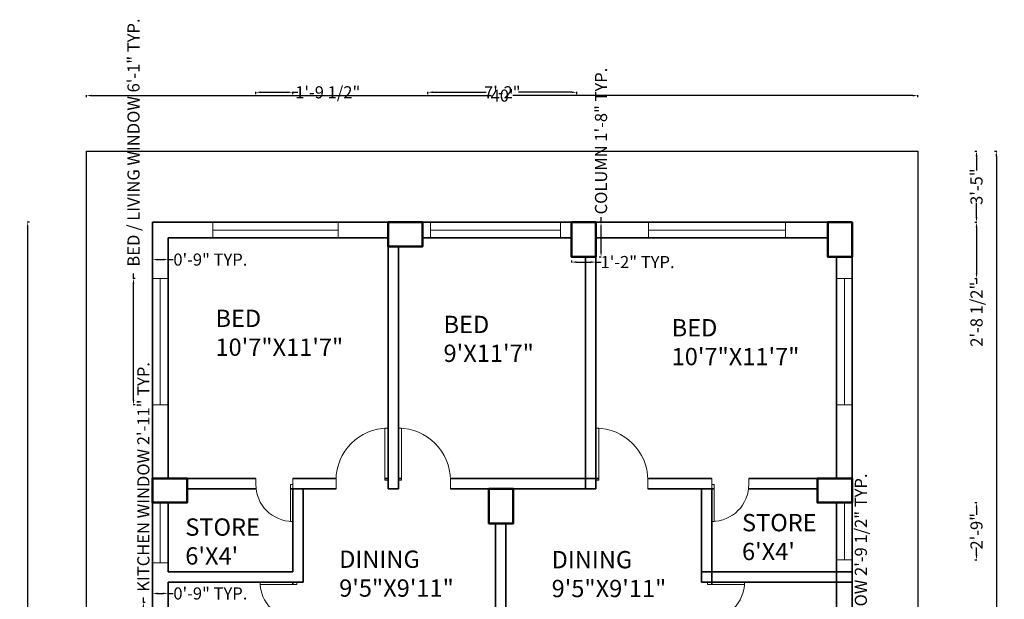
# Model space of a CAD drawing. Units: inches. Extents: x -78 to 529, y -573 to 148.
# Tile 2 of 2: x -78 to 491, y -187 to 148. Entities that reach past the tile are written whole.
import ezdxf

# ---------------------------------------------------------------- set-up
doc = ezdxf.new("R2010")
doc.units = ezdxf.units.IN
doc.header["$MEASUREMENT"] = 0
for name, color, linetype, lineweight in [('A-ANNO-DIMS', 2, 'Continuous', 18), ('A-AREA-IDEN', 5, 'Continuous', 18), ('A-COLS', 1, 'Continuous', 50), ('A-DOOR', 3, 'Continuous', 18), ('A-GLAZ', 4, 'Continuous', 18), ('A-WALL', 7, 'Continuous', 35), ('C-PROP', 8, 'Continuous', 25)]:
    doc.layers.add(name, color=color, linetype=linetype, lineweight=lineweight)
doc.styles.get("Standard").update_dxf_attribs({"font": 'arial.ttf'})
doc.dimstyles.get("Standard").update_dxf_attribs({"dimtxt": 7, "dimasz": 3, "dimexe": 0.18, "dimexo": 0.0625, "dimgap": 0.09, "dimtad": 0, "dimdec": 0, "dimzin": 0, "dimdsep": 46, "dimlunit": 3, "dimtxsty": 'Standard', "dimcen": 0.09, "dimadec": 0, "dimazin": 0, "dimtfac": 1, "dimtdec": 0, "dimtofl": 0, "dimtmove": 0, "dimatfit": 3, "dimfxl": 1, "dimfxlon": 1, "dimtolj": 1, "dimtzin": 0, "dimarcsym": 0})

# ---------------------------------------------------------------- blocks, each defined once
blk = doc.blocks.new('*U2')
for p, q in [((0, 0), (0, -5)), ((30, 0), (30, -5))]:
    blk.add_line(p, q)
blk.add_lwpolyline([(0, 0), (0, 30), (1.75, 30), (1.75, 0)], close=True)
blk.add_arc((0, 0), 30, 0, 90)
blk = doc.blocks.new('*D3')
at = {"layer": 'A-ANNO-DIMS', "color": 0, "lineweight": -2, "transparency": 16777216}
for p, q in [((-39.22, 102.81), (-39.22, 103.99)), ((-36.22, 103.81), (194.61, 103.81)), ((437.78, 103.81), (206.95, 103.81)), ((440.78, 102.81), (440.78, 103.99))]:
    blk.add_line(p, q, dxfattribs=at)
at = {"layer": 'A-ANNO-DIMS', "color": 0, "transparency": 16777216}
for points in [[(-36.22, 104.31), (-36.22, 103.31), (-39.22, 103.81)], [(437.78, 104.31), (437.78, 103.31), (440.78, 103.81)]]:
    blk.add_solid(points, dxfattribs=at)
at = {"layer": 'Defpoints', "color": 0, "transparency": 16777216}
for p in [(-39.22, 103.81), (-39.22, 71.78), (440.78, 71.78)]:
    blk.add_point(p, dxfattribs=at)
at = {"layer": 'A-ANNO-DIMS', "color": 0, "transparency": 16777216, "insert": (200.78, 103.81), "char_height": 7, "attachment_point": 5}
blk.add_mtext("\\A1;40'", dxfattribs=at)
blk = doc.blocks.new('*D4')
at = {"layer": 'A-ANNO-DIMS', "color": 0, "lineweight": -2, "transparency": 16777216}
for p, q in [((485.19, 71.78), (486.37, 71.78)), ((486.19, 68.78), (486.19, -222.19)), ((486.19, -525.22), (486.19, -234.25)), ((485.19, -528.22), (486.37, -528.22))]:
    blk.add_line(p, q, dxfattribs=at)
at = {"layer": 'A-ANNO-DIMS', "color": 0, "transparency": 16777216}
for points in [[(485.69, 68.78), (486.69, 68.78), (486.19, 71.78)], [(485.69, -525.22), (486.69, -525.22), (486.19, -528.22)]]:
    blk.add_solid(points, dxfattribs=at)
at = {"layer": 'Defpoints', "color": 0, "transparency": 16777216}
for p in [(440.78, 71.78), (440.78, -528.22), (486.19, -528.22)]:
    blk.add_point(p, dxfattribs=at)
at = {"layer": 'A-ANNO-DIMS', "color": 0, "transparency": 16777216, "insert": (486.19, -228.22), "char_height": 7, "attachment_point": 5, "rotation": 90}
blk.add_mtext("\\A1;50'", dxfattribs=at)
blk = doc.blocks.new('COLUMN-14X20')
blk.add_lwpolyline([(0, 20), (14, 20), (14, 0), (0, 0)], close=True)
blk = doc.blocks.new('WIN-BED-LIVING')
for p, q in [((0, 73.06), (9, 73.06)), ((4.5, 0), (4.5, 73.06)), ((0, 0), (9, 0))]:
    blk.add_line(p, q)
blk = doc.blocks.new('*D10')
at = {"layer": 'A-ANNO-DIMS', "color": 0, "lineweight": -2, "transparency": 16777216}
for p, q in [((256.91, 30.61), (258.09, 30.61)), ((257.91, 30.61), (257.91, 33.61)), ((257.91, 13.61), (257.91, 27.61)), ((256.91, 10.61), (258.09, 10.61))]:
    blk.add_line(p, q, dxfattribs=at)
at = {"layer": 'A-ANNO-DIMS', "color": 0, "transparency": 16777216}
for points in [[(257.41, 27.61), (258.41, 27.61), (257.91, 30.61)], [(257.41, 13.61), (258.41, 13.61), (257.91, 10.61)]]:
    blk.add_solid(points, dxfattribs=at)
at = {"layer": 'Defpoints', "color": 0, "transparency": 16777216}
for p in [(254.91, 30.61), (257.91, 30.61), (254.91, 10.61)]:
    blk.add_point(p, dxfattribs=at)
at = {"layer": 'A-ANNO-DIMS', "color": 0, "transparency": 16777216, "insert": (257.91, 77.54), "char_height": 7, "attachment_point": 5, "rotation": 90}
blk.add_mtext('\\A1;COLUMN 1\'-8" TYP.', dxfattribs=at)
blk = doc.blocks.new('*D11')
at = {"layer": 'A-ANNO-DIMS', "color": 0, "lineweight": -2, "transparency": 16777216}
for p, q in [((240.91, 8.61), (240.91, 7.43)), ((243.91, 7.61), (251.91, 7.61)), ((254.91, 8.61), (254.91, 7.43)), ((254.91, 7.61), (257.91, 7.61))]:
    blk.add_line(p, q, dxfattribs=at)
at = {"layer": 'A-ANNO-DIMS', "color": 0, "transparency": 16777216}
for points in [[(243.91, 8.11), (243.91, 7.11), (240.91, 7.61)], [(251.91, 8.11), (251.91, 7.11), (254.91, 7.61)]]:
    blk.add_solid(points, dxfattribs=at)
at = {"layer": 'Defpoints', "color": 0, "transparency": 16777216}
for p in [(240.91, 10.61), (254.91, 10.61), (254.91, 7.61)]:
    blk.add_point(p, dxfattribs=at)
at = {"layer": 'A-ANNO-DIMS', "color": 0, "transparency": 16777216, "insert": (279.01, 7.61), "char_height": 7, "attachment_point": 5}
blk.add_mtext('\\A1;1\'-2" TYP.', dxfattribs=at)
blk = doc.blocks.new('*D12')
at = {"layer": 'A-ANNO-DIMS', "color": 0, "lineweight": -2, "transparency": 16777216}
for p, q in [((-12.05, -1.91), (-12.05, 1.09)), ((-11.05, -1.91), (-12.23, -1.91)), ((-12.05, -71.97), (-12.05, -4.91)), ((-11.05, -74.97), (-12.23, -74.97))]:
    blk.add_line(p, q, dxfattribs=at)
at = {"layer": 'A-ANNO-DIMS', "color": 0, "transparency": 16777216}
for points in [[(-12.55, -4.91), (-11.55, -4.91), (-12.05, -1.91)], [(-12.55, -71.97), (-11.55, -71.97), (-12.05, -74.97)]]:
    blk.add_solid(points, dxfattribs=at)
at = {"layer": 'Defpoints', "color": 0, "transparency": 16777216}
for p in [(-12.05, -1.91), (-1.09, -1.91), (-1.09, -74.97)]:
    blk.add_point(p, dxfattribs=at)
at = {"layer": 'A-ANNO-DIMS', "color": 0, "transparency": 16777216, "insert": (-12.05, 76.69), "char_height": 7, "attachment_point": 5, "rotation": 90}
blk.add_mtext('\\A1;BED / LIVING WINDOW 6\'-1" TYP.', dxfattribs=at)
blk = doc.blocks.new('*D13')
at = {"layer": 'A-ANNO-DIMS', "color": 0, "lineweight": -2, "transparency": 16777216}
for p, q in [((-1.09, 8.05), (-1.09, 9.23)), ((1.91, 9.05), (4.91, 9.05)), ((7.91, 8.05), (7.91, 9.23)), ((7.91, 9.05), (10.91, 9.05))]:
    blk.add_line(p, q, dxfattribs=at)
at = {"layer": 'A-ANNO-DIMS', "color": 0, "transparency": 16777216}
for points in [[(1.91, 9.55), (1.91, 8.55), (-1.09, 9.05)], [(4.91, 9.55), (4.91, 8.55), (7.91, 9.05)]]:
    blk.add_solid(points, dxfattribs=at)
at = {"layer": 'Defpoints', "color": 0, "transparency": 16777216}
for p in [(7.91, 9.05), (-1.09, -1.91), (7.91, -1.91)]:
    blk.add_point(p, dxfattribs=at)
at = {"layer": 'A-ANNO-DIMS', "color": 0, "transparency": 16777216, "insert": (32.34, 9.05), "char_height": 7, "attachment_point": 5}
blk.add_mtext('\\A1;0\'-9" TYP.', dxfattribs=at)
blk = doc.blocks.new('*D16')
at = {"layer": 'A-ANNO-DIMS', "color": 0, "lineweight": -2, "transparency": 16777216}
for p, q in [((-6.35, -189.15), (-6.35, -186.15)), ((-5.35, -189.15), (-6.53, -189.15)), ((-6.35, -221.25), (-6.35, -192.15)), ((-5.35, -224.25), (-6.53, -224.25))]:
    blk.add_line(p, q, dxfattribs=at)
at = {"layer": 'A-ANNO-DIMS', "color": 0, "transparency": 16777216}
for points in [[(-6.85, -192.15), (-5.85, -192.15), (-6.35, -189.15)], [(-6.85, -221.25), (-5.85, -221.25), (-6.35, -224.25)]]:
    blk.add_solid(points, dxfattribs=at)
at = {"layer": 'Defpoints', "color": 0, "transparency": 16777216}
for p in [(-6.35, -189.15), (-1.09, -189.15), (-1.09, -224.25)]:
    blk.add_point(p, dxfattribs=at)
at = {"layer": 'A-ANNO-DIMS', "color": 0, "transparency": 16777216, "insert": (-6.35, -116.53), "char_height": 7, "attachment_point": 5, "rotation": 90}
blk.add_mtext('\\A1;KITCHEN WINDOW 2\'-11" TYP.', dxfattribs=at)
blk = doc.blocks.new('*D17')
at = {"layer": 'A-ANNO-DIMS', "color": 0, "lineweight": -2, "transparency": 16777216}
for p, q in [((-1.09, -184.89), (-1.09, -183.71)), ((1.91, -183.89), (4.91, -183.89)), ((7.91, -184.89), (7.91, -183.71)), ((7.91, -183.89), (10.91, -183.89))]:
    blk.add_line(p, q, dxfattribs=at)
at = {"layer": 'A-ANNO-DIMS', "color": 0, "transparency": 16777216}
for points in [[(1.91, -183.39), (1.91, -184.39), (-1.09, -183.89)], [(4.91, -183.39), (4.91, -184.39), (7.91, -183.89)]]:
    blk.add_solid(points, dxfattribs=at)
at = {"layer": 'Defpoints', "color": 0, "transparency": 16777216}
for p in [(7.91, -183.89), (-1.09, -189.15), (7.91, -189.15)]:
    blk.add_point(p, dxfattribs=at)
at = {"layer": 'A-ANNO-DIMS', "color": 0, "transparency": 16777216, "insert": (32.34, -183.89), "char_height": 7, "attachment_point": 5}
blk.add_mtext('\\A1;0\'-9" TYP.', dxfattribs=at)
blk = doc.blocks.new('*D18')
at = {"layer": 'A-ANNO-DIMS', "color": 0, "lineweight": -2, "transparency": 16777216}
for p, q in [((407.95, -256.39), (407.95, -253.39)), ((406.95, -256.39), (408.13, -256.39)), ((407.95, -286.96), (407.95, -259.39)), ((406.95, -289.96), (408.13, -289.96))]:
    blk.add_line(p, q, dxfattribs=at)
at = {"layer": 'A-ANNO-DIMS', "color": 0, "transparency": 16777216}
for points in [[(407.45, -259.39), (408.45, -259.39), (407.95, -256.39)], [(407.45, -286.96), (408.45, -286.96), (407.95, -289.96)]]:
    blk.add_solid(points, dxfattribs=at)
at = {"layer": 'Defpoints', "color": 0, "transparency": 16777216}
for p in [(402.91, -256.39), (407.95, -256.39), (402.91, -289.96)]:
    blk.add_point(p, dxfattribs=at)
at = {"layer": 'A-ANNO-DIMS', "color": 0, "transparency": 16777216, "insert": (407.95, -182.44), "char_height": 7, "attachment_point": 5, "rotation": 90}
blk.add_mtext('\\A1;TOILET WINDOW 2\'-9 1/2" TYP.', dxfattribs=at)
blk = doc.blocks.new('*D21')
at = {"layer": 'A-ANNO-DIMS', "color": 0, "lineweight": -2, "transparency": 16777216}
for p, q in [((-72.17, 30.61), (-73.35, 30.61)), ((-73.17, 27.61), (-73.17, -212.14)), ((-73.17, -476.39), (-73.17, -236.65)), ((-72.17, -479.39), (-73.35, -479.39))]:
    blk.add_line(p, q, dxfattribs=at)
at = {"layer": 'A-ANNO-DIMS', "color": 0, "transparency": 16777216}
for points in [[(-73.67, 27.61), (-72.67, 27.61), (-73.17, 30.61)], [(-73.67, -476.39), (-72.67, -476.39), (-73.17, -479.39)]]:
    blk.add_solid(points, dxfattribs=at)
at = {"layer": 'Defpoints', "color": 0, "transparency": 16777216}
for p in [(-73.17, 30.61), (-1.09, 30.61), (-1.09, -479.39)]:
    blk.add_point(p, dxfattribs=at)
at = {"layer": 'A-ANNO-DIMS', "color": 0, "transparency": 16777216, "insert": (-73.17, -224.39), "char_height": 7, "attachment_point": 5, "rotation": 90}
blk.add_mtext('\\A1;42\'-6"', dxfattribs=at)
blk = doc.blocks.new('*D23')
at = {"layer": 'A-ANNO-DIMS', "color": 0, "lineweight": -2, "transparency": 16777216}
for p, q in [((473.73, 71.78), (474.91, 71.78)), ((474.73, 68.78), (474.73, 60.59)), ((474.73, 33.61), (474.73, 41.8)), ((473.73, 30.61), (474.91, 30.61))]:
    blk.add_line(p, q, dxfattribs=at)
at = {"layer": 'A-ANNO-DIMS', "color": 0, "transparency": 16777216}
for points in [[(474.23, 68.78), (475.23, 68.78), (474.73, 71.78)], [(474.23, 33.61), (475.23, 33.61), (474.73, 30.61)]]:
    blk.add_solid(points, dxfattribs=at)
at = {"layer": 'Defpoints', "color": 0, "transparency": 16777216}
for p in [(440.78, 71.78), (402.91, 30.61), (474.73, 30.61)]:
    blk.add_point(p, dxfattribs=at)
at = {"layer": 'A-ANNO-DIMS', "color": 0, "transparency": 16777216, "insert": (474.73, 51.19), "char_height": 7, "attachment_point": 5, "rotation": 90}
blk.add_mtext('\\A1;3\'-5"', dxfattribs=at)
blk = doc.blocks.new('*D24')
at = {"layer": 'A-ANNO-DIMS', "color": 0, "lineweight": -2, "transparency": 16777216}
for p, q in [((157.91, 104.73), (157.91, 105.91)), ((160.91, 105.73), (191.55, 105.73)), ((240.91, 105.73), (210.28, 105.73)), ((243.91, 104.73), (243.91, 105.91))]:
    blk.add_line(p, q, dxfattribs=at)
at = {"layer": 'A-ANNO-DIMS', "color": 0, "transparency": 16777216}
for points in [[(160.91, 106.23), (160.91, 105.23), (157.91, 105.73)], [(240.91, 106.23), (240.91, 105.23), (243.91, 105.73)]]:
    blk.add_solid(points, dxfattribs=at)
at = {"layer": 'Defpoints', "color": 0, "transparency": 16777216}
for p in [(243.91, 105.73), (157.91, -433.39), (243.91, -433.39)]:
    blk.add_point(p, dxfattribs=at)
at = {"layer": 'A-ANNO-DIMS', "color": 0, "transparency": 16777216, "insert": (200.91, 105.73), "char_height": 7, "attachment_point": 5}
blk.add_mtext('\\A1;7\'-2"', dxfattribs=at)
blk = doc.blocks.new('*D28')
at = {"layer": 'A-ANNO-DIMS', "color": 0, "lineweight": -2, "transparency": 16777216}
for p, q in [((58.59, 104.73), (58.59, 105.91)), ((61.59, 105.73), (76.91, 105.73)), ((79.91, 104.73), (79.91, 105.91)), ((79.91, 105.73), (82.91, 105.73))]:
    blk.add_line(p, q, dxfattribs=at)
at = {"layer": 'A-ANNO-DIMS', "color": 0, "transparency": 16777216}
for points in [[(61.59, 106.23), (61.59, 105.23), (58.59, 105.73)], [(76.91, 106.23), (76.91, 105.23), (79.91, 105.73)]]:
    blk.add_solid(points, dxfattribs=at)
at = {"layer": 'Defpoints', "color": 0, "transparency": 16777216}
for p in [(79.91, 105.73), (58.59, -117.39), (79.91, -117.39)]:
    blk.add_point(p, dxfattribs=at)
at = {"layer": 'A-ANNO-DIMS', "color": 0, "transparency": 16777216, "insert": (100.13, 105.73), "char_height": 7, "attachment_point": 5}
blk.add_mtext('\\A1;1\'-9 1/2"', dxfattribs=at)
blk = doc.blocks.new('*D29')
at = {"layer": 'A-ANNO-DIMS', "color": 0, "lineweight": -2, "transparency": 16777216}
for p, q in [((7.91, -561.17), (7.91, -562.35)), ((10.91, -562.17), (11.34, -562.17)), ((30.68, -562.17), (30.25, -562.17)), ((33.68, -561.17), (33.68, -562.35))]:
    blk.add_line(p, q, dxfattribs=at)
at = {"layer": 'A-ANNO-DIMS', "color": 0, "transparency": 16777216}
for points in [[(10.91, -561.67), (10.91, -562.67), (7.91, -562.17)], [(30.68, -561.67), (30.68, -562.67), (33.68, -562.17)]]:
    blk.add_solid(points, dxfattribs=at)
at = {"layer": 'Defpoints', "color": 0, "transparency": 16777216}
for p in [(7.91, 21.61), (33.68, 21.61), (33.68, -562.17)]:
    blk.add_point(p, dxfattribs=at)
at = {"layer": 'A-ANNO-DIMS', "color": 0, "transparency": 16777216, "insert": (20.79, -562.17), "char_height": 7, "attachment_point": 5}
blk.add_mtext('\\A1;2\'-2"', dxfattribs=at)
blk = doc.blocks.new('*D30')
at = {"layer": 'A-ANNO-DIMS', "color": 0, "lineweight": -2, "transparency": 16777216}
for p, q in [((33.68, -561.17), (33.68, -562.35)), ((36.68, -562.17), (52.37, -562.17)), ((103.2, -562.17), (87.51, -562.17)), ((106.2, -561.17), (106.2, -562.35))]:
    blk.add_line(p, q, dxfattribs=at)
at = {"layer": 'A-ANNO-DIMS', "color": 0, "transparency": 16777216}
for points in [[(36.68, -561.67), (36.68, -562.67), (33.68, -562.17)], [(103.2, -561.67), (103.2, -562.67), (106.2, -562.17)]]:
    blk.add_solid(points, dxfattribs=at)
at = {"layer": 'Defpoints', "color": 0, "transparency": 16777216}
for p in [(33.68, 21.61), (106.2, 21.61), (106.2, -562.17)]:
    blk.add_point(p, dxfattribs=at)
at = {"layer": 'A-ANNO-DIMS', "color": 0, "transparency": 16777216, "insert": (69.94, -562.17), "char_height": 7, "attachment_point": 5}
blk.add_mtext('\\A1;6\'-0 1/2"', dxfattribs=at)
blk = doc.blocks.new('*D31')
at = {"layer": 'A-ANNO-DIMS', "color": 0, "lineweight": -2, "transparency": 16777216}
for p, q in [((134.91, -561.17), (134.91, -562.35)), ((137.91, -562.17), (156.38, -562.17)), ((159.38, -561.17), (159.38, -562.35)), ((159.38, -562.17), (162.38, -562.17))]:
    blk.add_line(p, q, dxfattribs=at)
at = {"layer": 'A-ANNO-DIMS', "color": 0, "transparency": 16777216}
for points in [[(137.91, -561.67), (137.91, -562.67), (134.91, -562.17)], [(156.38, -561.67), (156.38, -562.67), (159.38, -562.17)]]:
    blk.add_solid(points, dxfattribs=at)
at = {"layer": 'Defpoints', "color": 0, "transparency": 16777216}
for p in [(134.91, 30.61), (159.38, 21.61), (159.38, -562.17)]:
    blk.add_point(p, dxfattribs=at)
at = {"layer": 'A-ANNO-DIMS', "color": 0, "transparency": 16777216, "insert": (179.99, -562.17), "char_height": 7, "attachment_point": 5}
blk.add_mtext('\\A1;2\'-0 1/2"', dxfattribs=at)
blk = doc.blocks.new('*D32')
at = {"layer": 'A-ANNO-DIMS', "color": 0, "lineweight": -2, "transparency": 16777216}
for p, q in [((159.38, -561.17), (159.38, -562.35)), ((162.38, -562.17), (187.51, -562.17)), ((231.46, -562.17), (206.34, -562.17)), ((234.46, -561.17), (234.46, -562.35))]:
    blk.add_line(p, q, dxfattribs=at)
at = {"layer": 'A-ANNO-DIMS', "color": 0, "transparency": 16777216}
for points in [[(162.38, -561.67), (162.38, -562.67), (159.38, -562.17)], [(231.46, -561.67), (231.46, -562.67), (234.46, -562.17)]]:
    blk.add_solid(points, dxfattribs=at)
at = {"layer": 'Defpoints', "color": 0, "transparency": 16777216}
for p in [(159.38, 21.61), (234.46, 21.61), (234.46, -562.17)]:
    blk.add_point(p, dxfattribs=at)
at = {"layer": 'A-ANNO-DIMS', "color": 0, "transparency": 16777216, "insert": (196.92, -562.17), "char_height": 7, "attachment_point": 5}
blk.add_mtext('\\A1;6\'-3"', dxfattribs=at)
blk = doc.blocks.new('*D33')
at = {"layer": 'A-ANNO-DIMS', "color": 0, "lineweight": -2, "transparency": 16777216}
for p, q in [((364.5, -561.17), (364.5, -562.35)), ((367.5, -562.17), (385.91, -562.17)), ((388.91, -561.17), (388.91, -562.35)), ((388.91, -562.17), (391.91, -562.17))]:
    blk.add_line(p, q, dxfattribs=at)
at = {"layer": 'A-ANNO-DIMS', "color": 0, "transparency": 16777216}
for points in [[(367.5, -561.67), (367.5, -562.67), (364.5, -562.17)], [(385.91, -561.67), (385.91, -562.67), (388.91, -562.17)]]:
    blk.add_solid(points, dxfattribs=at)
at = {"layer": 'Defpoints', "color": 0, "transparency": 16777216}
for p in [(364.5, 21.61), (388.91, 10.61), (388.91, -562.17)]:
    blk.add_point(p, dxfattribs=at)
at = {"layer": 'A-ANNO-DIMS', "color": 0, "transparency": 16777216, "insert": (409.52, -562.17), "char_height": 7, "attachment_point": 5}
blk.add_mtext('\\A1;2\'-0 1/2"', dxfattribs=at)
blk = doc.blocks.new('*D34')
at = {"layer": 'A-ANNO-DIMS', "color": 0, "lineweight": -2, "transparency": 16777216}
for p, q in [((285.28, -561.17), (285.28, -562.35)), ((288.28, -562.17), (315.48, -562.17)), ((361.5, -562.17), (334.3, -562.17)), ((364.5, -561.17), (364.5, -562.35))]:
    blk.add_line(p, q, dxfattribs=at)
at = {"layer": 'A-ANNO-DIMS', "color": 0, "transparency": 16777216}
for points in [[(288.28, -561.67), (288.28, -562.67), (285.28, -562.17)], [(361.5, -561.67), (361.5, -562.67), (364.5, -562.17)]]:
    blk.add_solid(points, dxfattribs=at)
at = {"layer": 'Defpoints', "color": 0, "transparency": 16777216}
for p in [(285.28, 21.61), (364.5, 21.61), (364.5, -562.17)]:
    blk.add_point(p, dxfattribs=at)
at = {"layer": 'A-ANNO-DIMS', "color": 0, "transparency": 16777216, "insert": (324.89, -562.17), "char_height": 7, "attachment_point": 5}
blk.add_mtext('\\A1;6\'-7"', dxfattribs=at)
blk = doc.blocks.new('*D35')
at = {"layer": 'A-ANNO-DIMS', "color": 0, "lineweight": -2, "transparency": 16777216}
for p, q in [((473.73, 30.61), (474.91, 30.61)), ((474.73, 27.61), (474.73, 1.09)), ((473.73, -1.91), (474.91, -1.91)), ((474.73, -1.91), (474.73, -4.91))]:
    blk.add_line(p, q, dxfattribs=at)
at = {"layer": 'A-ANNO-DIMS', "color": 0, "transparency": 16777216}
for points in [[(474.23, 27.61), (475.23, 27.61), (474.73, 30.61)], [(474.23, 1.09), (475.23, 1.09), (474.73, -1.91)]]:
    blk.add_solid(points, dxfattribs=at)
at = {"layer": 'Defpoints', "color": 0, "transparency": 16777216}
for p in [(402.91, 30.61), (402.91, -1.91), (474.73, -1.91)]:
    blk.add_point(p, dxfattribs=at)
at = {"layer": 'A-ANNO-DIMS', "color": 0, "transparency": 16777216, "insert": (474.73, -22.52), "char_height": 7, "attachment_point": 5, "rotation": 90}
blk.add_mtext('\\A1;2\'-8 1/2"', dxfattribs=at)
blk = doc.blocks.new('*D37')
at = {"layer": 'A-ANNO-DIMS', "color": 0, "lineweight": -2, "transparency": 16777216}
for p, q in [((473.73, -131.41), (474.91, -131.41)), ((474.73, -134.41), (474.73, -138.48)), ((474.73, -161.46), (474.73, -157.39)), ((473.73, -164.46), (474.91, -164.46))]:
    blk.add_line(p, q, dxfattribs=at)
at = {"layer": 'A-ANNO-DIMS', "color": 0, "transparency": 16777216}
for points in [[(474.23, -134.41), (475.23, -134.41), (474.73, -131.41)], [(474.23, -161.46), (475.23, -161.46), (474.73, -164.46)]]:
    blk.add_solid(points, dxfattribs=at)
at = {"layer": 'Defpoints', "color": 0, "transparency": 16777216}
for p in [(402.91, -131.41), (402.91, -164.46), (474.73, -164.46)]:
    blk.add_point(p, dxfattribs=at)
at = {"layer": 'A-ANNO-DIMS', "color": 0, "transparency": 16777216, "insert": (474.73, -147.94), "char_height": 7, "attachment_point": 5, "rotation": 90}
blk.add_mtext('\\A1;2\'-9"', dxfattribs=at)
blk = doc.blocks.new('*D38')
at = {"layer": 'A-ANNO-DIMS', "color": 0, "lineweight": -2, "transparency": 16777216}
for p, q in [((131.91, -562.17), (128.91, -562.17)), ((134.91, -561.17), (134.91, -562.35)), ((140.91, -561.17), (140.91, -562.35)), ((143.91, -562.17), (146.91, -562.17))]:
    blk.add_line(p, q, dxfattribs=at)
at = {"layer": 'A-ANNO-DIMS', "color": 0, "transparency": 16777216}
for points in [[(131.91, -561.67), (131.91, -562.67), (134.91, -562.17)], [(143.91, -561.67), (143.91, -562.67), (140.91, -562.17)]]:
    blk.add_solid(points, dxfattribs=at)
at = {"layer": 'Defpoints', "color": 0, "transparency": 16777216}
for p in [(134.91, -123.39), (140.91, -123.39), (140.91, -562.17)]:
    blk.add_point(p, dxfattribs=at)
at = {"layer": 'A-ANNO-DIMS', "color": 0, "transparency": 16777216, "insert": (156.31, -562.17), "char_height": 7, "attachment_point": 5}
blk.add_mtext('\\A1;0\'-6"', dxfattribs=at)

msp = doc.modelspace()

# ---------------------------------------------------------------- linework, layer by layer
at = {"layer": 'A-GLAZ'}
for p, q in [((33.68, 30.61), (33.68, 21.61)), ((106.2, 30.61), (106.2, 21.61)), ((159.38, 30.61), (159.38, 21.61)), ((234.46, 30.61), (234.46, 21.61)), ((285.28, 30.61), (285.28, 21.61)), ((364.5, 30.61), (364.5, 21.61)), ((33.68, 26.11), (106.2, 26.11)), ((159.38, 26.11), (234.46, 26.11)), ((285.28, 26.11), (364.5, 26.11)), ((3.41, -131.39), (3.41, -166.28)), ((398.41, -131.41), (398.41, -164.46)), ((393.91, -164.46), (402.91, -164.46)), ((-1.09, -166.28), (7.91, -166.28))]:
    msp.add_line(p, q, dxfattribs=at)
at = {"layer": 'A-WALL'}
for p, q in [((-1.09, 30.61), (402.91, 30.61)), ((-1.09, 30.61), (-1.09, -439.39)), ((402.91, 30.61), (402.91, -439.39)), ((7.91, 21.61), (134.91, 21.61)), ((7.91, 21.61), (7.91, -117.39)), ((134.91, 21.61), (134.91, -123.39)), ((154.91, 21.61), (240.91, 21.61)), ((254.91, 21.61), (254.91, -123.39)), ((254.91, 21.61), (388.91, 21.61)), ((140.91, 16.61), (140.91, -123.39)), ((248.91, 10.61), (248.91, -123.39)), ((393.91, 10.61), (393.91, -117.39)), ((7.91, -117.39), (58.59, -117.39)), ((79.91, -117.39), (104.93, -117.39)), ((133.16, -117.39), (134.91, -117.39)), ((140.91, -117.39), (142.66, -117.39)), ((170.89, -117.39), (256.66, -117.39)), ((284.89, -117.39), (321.91, -117.39)), ((343.23, -117.39), (393.91, -117.39)), ((18.91, -123.39), (58.73, -123.39)), ((78.67, -123.39), (104.91, -123.39)), ((79.91, -123.39), (79.91, -171.39)), ((85.91, -123.39), (85.91, -177.39)), ((134.91, -123.39), (140.91, -123.39)), ((170.91, -123.39), (254.91, -123.39)), ((284.91, -123.39), (323.15, -123.39)), ((315.91, -123.39), (315.91, -177.39)), ((321.91, -123.39), (321.91, -178.64)), ((343.09, -123.39), (382.91, -123.39)), ((7.91, -131.39), (7.91, -171.39)), ((393.91, -131.41), (393.91, -242.39)), ((196.91, -143.39), (196.91, -242.39)), ((202.91, -143.39), (202.91, -242.39)), ((7.91, -171.39), (79.91, -171.39)), ((315.91, -171.39), (402.91, -171.39)), ((7.91, -177.39), (85.91, -177.39)), ((7.91, -177.39), (7.91, -242.39)), ((79.91, -177.39), (79.91, -178.64)), ((315.91, -177.39), (402.91, -177.39))]:
    msp.add_line(p, q, dxfattribs=at)
at = {"layer": 'C-PROP'}
msp.add_lwpolyline([(-39.22, 71.78), (440.78, 71.78), (440.78, -528.22), (-39.22, -528.22)], close=True, dxfattribs=at)

# ---------------------------------------------------------------- block references
at = {"layer": 'A-COLS'}
for p, rotation in [((134.91, 30.61), 270), ((-1.09, -117.39), 270.0000000000001), ((382.91, -117.41), 270.0000000000001)]:
    msp.add_blockref('COLUMN-14X20', p, dxfattribs=dict(at, rotation=rotation))
for p in [(240.91, 10.61), (388.91, 10.61), (193.19, -143.39)]:
    msp.add_blockref('COLUMN-14X20', p, dxfattribs=at)
at = {"layer": 'A-DOOR', "xscale": -1}
msp.add_blockref('*U2', (134.91, -118.39), dxfattribs=at)
at = {"layer": 'A-DOOR'}
for p in [(140.91, -118.39), (254.91, -118.39)]:
    msp.add_blockref('*U2', p, dxfattribs=at)
at = {"layer": 'A-DOOR', "yscale": 0.710672036818973, "zscale": 0.710672036818973}
for p, xscale, rotation in [((79.91, -120.95), 0.710672036818973, 180), ((321.91, -120.95), -0.710672036818973, 180), ((82.36, -177.39), -0.710672036818973, 90), ((319.46, -177.39), 0.710672036818973, 270)]:
    msp.add_blockref('*U2', p, dxfattribs=dict(at, xscale=xscale, rotation=rotation))
at = {"layer": 'A-GLAZ'}
for p in [(-1.09, -74.97), (393.91, -74.97)]:
    msp.add_blockref('WIN-BED-LIVING', p, dxfattribs=at)

# ---------------------------------------------------------------- texts
at = {"layer": 'A-AREA-IDEN', "char_height": 10, "attachment_point": 1}
for s, insert in [('BED\\P10\'7"X11\'7"', (35.28, -19.91)), ('BED\\P9\'X11\'7"', (166.99, -23.43)), ('BED\\P10\'7"X11\'7"', (298.69, -25.34)), ("STORE\\P6'X4'", (17.86, -140.53)), ("STORE\\P6'X4'", (339.32, -137.97)), ('DINING\\P9\'5"X9\'11"', (106.72, -159.1)), ('DINING\\P9\'5"X9\'11"', (229.39, -159.36))]:
    msp.add_mtext_dynamic_manual_height_columns(s, width=71.5571, gutter_width=1, heights=[0], dxfattribs=dict(at, insert=insert))

# ---------------------------------------------------------------- dimensions: what is measured, and where the dimension line sits
at = {"layer": 'A-ANNO-DIMS'}
for base, p1, p2, text, picture, middle in [((-12.05, -1.91), (-1.09, -74.97), (-1.09, -1.91), 'BED / LIVING WINDOW <> TYP.', '*D12', (-12.05, 76.69)), ((257.91, 30.61), (254.91, 10.61), (254.91, 30.61), 'COLUMN <> TYP.', '*D10', (257.91, 77.54)), ((-6.35, -189.15), (-1.09, -224.25), (-1.09, -189.15), 'KITCHEN WINDOW <> TYP.', '*D16', (-6.35, -116.53)), ((407.95, -256.39), (402.91, -289.96), (402.91, -256.39), 'TOILET WINDOW <> TYP.', '*D18', (407.95, -182.44))]:
    dim = msp.add_linear_dim(base=base, p1=p1, p2=p2, angle=90, text=text, dimstyle='Standard', override={"dimdec": 1, "dimlfac": 1, "dimrnd": 0, "dimzin": 1, "dimdsep": 46, "dimlunit": 4, "dimfrac": 2}, dxfattribs=at)
    dim.commit()
    dim.dimension.update_dxf_attribs({"geometry": picture, "text_midpoint": middle})
for base, p1, p2, override, picture, middle in [((79.91, 105.73), (58.59, -117.39), (79.91, -117.39), {"dimdec": 1, "dimlfac": 1, "dimrnd": 0, "dimzin": 1, "dimdsep": 46, "dimlunit": 4, "dimfrac": 2}, '*D28', (100.13, 105.73)), ((-39.22, 103.81), (440.78, 71.78), (-39.22, 71.78), {"dimclrd": 0, "dimclre": 0, "dimclrt": 0}, '*D3', (200.78, 103.81)), ((243.91, 105.73), (157.91, -433.39), (243.91, -433.39), {"dimdec": 1, "dimlfac": 1, "dimrnd": 0, "dimzin": 1, "dimdsep": 46, "dimlunit": 4, "dimfrac": 2}, '*D24', (200.91, 105.73)), ((159.38, -562.17), (134.91, 30.61), (159.38, 21.61), {"dimdec": 1, "dimlfac": 1, "dimrnd": 0, "dimzin": 1, "dimdsep": 46, "dimlunit": 4, "dimfrac": 2}, '*D31', (179.99, -562.17)), ((33.68, -562.17), (7.91, 21.61), (33.68, 21.61), {"dimdec": 1, "dimlfac": 1, "dimrnd": 0, "dimzin": 1, "dimdsep": 46, "dimlunit": 4, "dimfrac": 2}, '*D29', (20.79, -562.17)), ((106.2, -562.17), (33.68, 21.61), (106.2, 21.61), {"dimdec": 1, "dimlfac": 1, "dimrnd": 0, "dimzin": 1, "dimdsep": 46, "dimlunit": 4, "dimfrac": 2}, '*D30', (69.94, -562.17)), ((234.46, -562.17), (159.38, 21.61), (234.46, 21.61), {"dimdec": 1, "dimlfac": 1, "dimrnd": 0, "dimzin": 1, "dimdsep": 46, "dimlunit": 4, "dimfrac": 2}, '*D32', (196.92, -562.17)), ((364.5, -562.17), (285.28, 21.61), (364.5, 21.61), {"dimdec": 1, "dimlfac": 1, "dimrnd": 0, "dimzin": 1, "dimdsep": 46, "dimlunit": 4, "dimfrac": 2}, '*D34', (324.89, -562.17)), ((388.91, -562.17), (364.5, 21.61), (388.91, 10.61), {"dimdec": 1, "dimlfac": 1, "dimrnd": 0, "dimzin": 1, "dimdsep": 46, "dimlunit": 4, "dimfrac": 2}, '*D33', (409.52, -562.17)), ((140.91, -562.17), (134.91, -123.39), (140.91, -123.39), {"dimdec": 1, "dimlfac": 1, "dimrnd": 0, "dimzin": 1, "dimdsep": 46, "dimlunit": 4, "dimfrac": 2}, '*D38', (156.31, -562.17))]:
    dim = msp.add_linear_dim(base=base, p1=p1, p2=p2, dimstyle='Standard', override=override, dxfattribs=at)
    dim.commit()
    dim.dimension.update_dxf_attribs({"geometry": picture, "text_midpoint": middle})
for base, p1, p2, override, picture, middle in [((474.73, 30.61), (440.78, 71.78), (402.91, 30.61), {"dimdec": 1, "dimlfac": 1, "dimrnd": 0, "dimzin": 1, "dimdsep": 46, "dimlunit": 4, "dimfrac": 2}, '*D23', (474.73, 51.19)), ((486.19, -528.22), (440.78, 71.78), (440.78, -528.22), {"dimclrd": 0, "dimclre": 0, "dimclrt": 0}, '*D4', (486.19, -228.22)), ((-73.17, 30.61), (-1.09, -479.39), (-1.09, 30.61), {"dimdec": 1, "dimlfac": 1, "dimrnd": 0, "dimzin": 1, "dimdsep": 46, "dimlunit": 4, "dimfrac": 2}, '*D21', (-73.17, -224.39)), ((474.73, -1.91), (402.91, 30.61), (402.91, -1.91), {"dimdec": 1, "dimlfac": 1, "dimrnd": 0, "dimzin": 1, "dimdsep": 46, "dimlunit": 4, "dimfrac": 2}, '*D35', (474.73, -22.52)), ((474.7332, -164.4636), (402.9113, -131.409), (402.9113, -164.4636), {"dimdec": 1, "dimlfac": 1, "dimrnd": 0, "dimzin": 1, "dimdsep": 46, "dimlunit": 4, "dimfrac": 2}, '*D37', (474.7332, -147.9363))]:
    dim = msp.add_linear_dim(base=base, p1=p1, p2=p2, angle=90, dimstyle='Standard', override=override, dxfattribs=at)
    dim.commit()
    dim.dimension.update_dxf_attribs({"geometry": picture, "text_midpoint": middle})
for base, p1, p2, picture, middle in [((7.91, 9.05), (-1.09, -1.91), (7.91, -1.91), '*D13', (32.34, 9.05)), ((254.91, 7.61), (240.91, 10.61), (254.91, 10.61), '*D11', (279.01, 7.61)), ((7.91, -183.89), (-1.09, -189.15), (7.91, -189.15), '*D17', (32.34, -183.89))]:
    dim = msp.add_linear_dim(base=base, p1=p1, p2=p2, text='<> TYP.', dimstyle='Standard', override={"dimdec": 1, "dimlfac": 1, "dimrnd": 0, "dimzin": 1, "dimdsep": 46, "dimlunit": 4, "dimfrac": 2}, dxfattribs=at)
    dim.commit()
    dim.dimension.update_dxf_attribs({"geometry": picture, "text_midpoint": middle})

doc.saveas('drawing.dxf')
